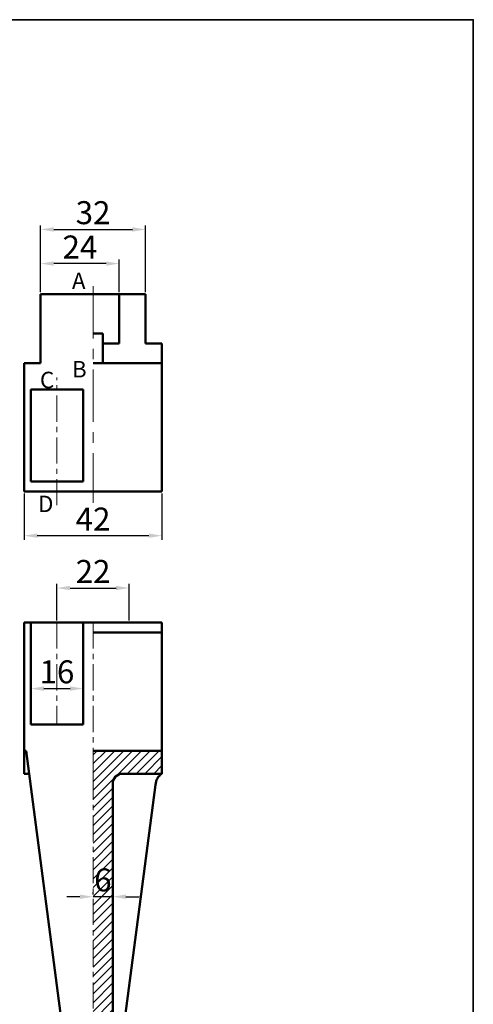
# Model space of a CAD drawing. Units: millimetres. Extents: x 214 to 813, y -258 to 321.
# Tile 4 of 4: x 674 to 813, y 22 to 321. Entities that reach past the tile are written whole.
import ezdxf

# ---------------------------------------------------------------- set-up
doc = ezdxf.new("R2010")
doc.units = ezdxf.units.MM
doc.header["$LTSCALE"] = 0.5
doc.linetypes.add('CENTER', pattern=[50.8, 31.75, -6.35, 6.35, -6.35])
for name, color, linetype, lineweight in [('M-CNTR', 1, 'CENTER', 18), ('M-DIMS', 2, 'Continuous', 25), ('M-HATC', 8, 'Continuous', 18), ('M-OUTL', 7, 'Continuous', 50), ('M-TEXT', 3, 'Continuous', 25), ('M-TTLB', 7, 'Continuous', 35)]:
    doc.layers.add(name, color=color, linetype=linetype, lineweight=lineweight)
doc.styles.get("Standard").update_dxf_attribs({"font": 'arial.ttf'})
doc.dimstyles.new('ISO-25', dxfattribs={"dimtxt": 7, "dimasz": 4, "dimexe": 1.25, "dimexo": 0.625, "dimtad": 1, "dimtoh": 1, "dimtxsty": 'Standard', "dimcen": 2.5, "dimadec": 0, "dimazin": 0, "dimtfac": 1, "dimtmove": 0, "dimatfit": 3, "dimfxl": 1, "dimarcsym": 0})

# ---------------------------------------------------------------- blocks, each defined once
blk = doc.blocks.new('*U58')
at = {"layer": 'M-CNTR', "color": 0, "transparency": 16777216}
blk.add_line((0, 41.44), (0, -24.5), dxfattribs=at)
blk = doc.blocks.new('*D59')
at = {"layer": 'Defpoints', "color": 0, "ltscale": 0.5, "transparency": 16777216}
for p in [(707.86, 148.54), (685.86, 138.04), (707.86, 138.04)]:
    blk.add_point(p, dxfattribs=at)
at = {"layer": 'M-DIMS', "color": 0, "lineweight": -2, "ltscale": 0.5, "transparency": 16777216}
for p, q in [((685.86, 138.67), (685.86, 149.79)), ((689.86, 148.54), (703.86, 148.54)), ((707.86, 138.67), (707.86, 149.79))]:
    blk.add_line(p, q, dxfattribs=at)
at = {"layer": 'M-DIMS', "color": 0, "ltscale": 0.5, "transparency": 16777216}
for points in [[(689.86, 149.21), (689.86, 147.88), (685.86, 148.54)], [(703.86, 149.21), (703.86, 147.88), (707.86, 148.54)]]:
    blk.add_solid(points, dxfattribs=at)
at = {"layer": 'M-DIMS', "color": 0, "ltscale": 0.5, "transparency": 16777216, "insert": (696.86, 152.68), "char_height": 7, "attachment_point": 5}
blk.add_mtext('22', dxfattribs=at)
blk = doc.blocks.new('*D60')
at = {"layer": 'Defpoints', "color": 0, "ltscale": 0.5, "transparency": 16777216}
for p in [(677.86, 117.94), (693.86, 117.94), (693.86, 117.94)]:
    blk.add_point(p, dxfattribs=at)
at = {"layer": 'M-DIMS', "color": 0, "lineweight": -2, "ltscale": 0.5, "transparency": 16777216}
for p, q in [((677.86, 118.56), (677.86, 119.19)), ((681.86, 117.94), (689.86, 117.94)), ((693.86, 118.56), (693.86, 119.19))]:
    blk.add_line(p, q, dxfattribs=at)
at = {"layer": 'M-DIMS', "color": 0, "ltscale": 0.5, "transparency": 16777216}
for points in [[(681.86, 118.6), (681.86, 117.27), (677.86, 117.94)], [(689.86, 118.6), (689.86, 117.27), (693.86, 117.94)]]:
    blk.add_solid(points, dxfattribs=at)
at = {"layer": 'M-DIMS', "color": 0, "ltscale": 0.5, "transparency": 16777216, "insert": (685.86, 122.13), "char_height": 7, "attachment_point": 5}
blk.add_mtext('16', dxfattribs=at)
blk = doc.blocks.new('*D61')
at = {"layer": 'Defpoints', "color": 0, "ltscale": 0.5, "transparency": 16777216}
for p in [(696.86, 54.6), (696.86, 54.6), (702.86, 54.6)]:
    blk.add_point(p, dxfattribs=at)
at = {"layer": 'M-DIMS', "color": 0, "lineweight": -2, "ltscale": 0.5, "transparency": 16777216}
for p, q in [((692.86, 54.6), (688.86, 54.6)), ((696.86, 55.23), (696.86, 55.85)), ((702.86, 54.6), (696.86, 54.6)), ((702.86, 55.23), (702.86, 55.85)), ((706.86, 54.6), (710.86, 54.6))]:
    blk.add_line(p, q, dxfattribs=at)
at = {"layer": 'M-DIMS', "color": 0, "ltscale": 0.5, "transparency": 16777216}
for points in [[(692.86, 55.27), (692.86, 53.94), (696.86, 54.6)], [(706.86, 55.27), (706.86, 53.94), (702.86, 54.6)]]:
    blk.add_solid(points, dxfattribs=at)
at = {"layer": 'M-DIMS', "color": 0, "ltscale": 0.5, "transparency": 16777216, "insert": (699.86, 58.8), "char_height": 7, "attachment_point": 5}
blk.add_mtext('6', dxfattribs=at)
blk = doc.blocks.new('*D66')
at = {"layer": 'Defpoints', "color": 0, "ltscale": 0.5, "transparency": 16777216}
for p in [(675.86, 177.96), (717.86, 177.96), (717.86, 164.48)]:
    blk.add_point(p, dxfattribs=at)
at = {"layer": 'M-DIMS', "color": 0, "lineweight": -2, "ltscale": 0.5, "transparency": 16777216}
for p, q in [((675.86, 177.34), (675.86, 163.23)), ((717.86, 177.34), (717.86, 163.23)), ((679.86, 164.48), (713.86, 164.48))]:
    blk.add_line(p, q, dxfattribs=at)
at = {"layer": 'M-DIMS', "color": 0, "ltscale": 0.5, "transparency": 16777216}
for points in [[(679.86, 165.14), (679.86, 163.81), (675.86, 164.48)], [(713.86, 165.14), (713.86, 163.81), (717.86, 164.48)]]:
    blk.add_solid(points, dxfattribs=at)
at = {"layer": 'M-DIMS', "color": 0, "ltscale": 0.5, "transparency": 16777216, "insert": (696.86, 168.62), "char_height": 7, "attachment_point": 5}
blk.add_mtext('42', dxfattribs=at)
blk = doc.blocks.new('*D67')
at = {"layer": 'Defpoints', "color": 0, "ltscale": 0.5, "transparency": 16777216}
for p in [(712.86, 257.66), (680.86, 237.96), (712.86, 237.96)]:
    blk.add_point(p, dxfattribs=at)
at = {"layer": 'M-DIMS', "color": 0, "lineweight": -2, "ltscale": 0.5, "transparency": 16777216}
for p, q in [((680.86, 238.59), (680.86, 258.91)), ((712.86, 238.59), (712.86, 258.91)), ((684.86, 257.66), (708.86, 257.66))]:
    blk.add_line(p, q, dxfattribs=at)
at = {"layer": 'M-DIMS', "color": 0, "ltscale": 0.5, "transparency": 16777216}
for points in [[(684.86, 258.33), (684.86, 256.99), (680.86, 257.66)], [(708.86, 258.33), (708.86, 256.99), (712.86, 257.66)]]:
    blk.add_solid(points, dxfattribs=at)
at = {"layer": 'M-DIMS', "color": 0, "ltscale": 0.5, "transparency": 16777216, "insert": (696.86, 261.86), "char_height": 7, "attachment_point": 5}
blk.add_mtext('32', dxfattribs=at)
blk = doc.blocks.new('*D68')
at = {"layer": 'Defpoints', "color": 0, "ltscale": 0.5, "transparency": 16777216}
for p in [(680.86, 247.28), (680.86, 237.96), (704.86, 237.96)]:
    blk.add_point(p, dxfattribs=at)
at = {"layer": 'M-DIMS', "color": 0, "lineweight": -2, "ltscale": 0.5, "transparency": 16777216}
for p, q in [((680.86, 238.59), (680.86, 248.53)), ((700.86, 247.28), (684.86, 247.28)), ((704.86, 238.59), (704.86, 248.53))]:
    blk.add_line(p, q, dxfattribs=at)
at = {"layer": 'M-DIMS', "color": 0, "ltscale": 0.5, "transparency": 16777216}
for points in [[(684.86, 247.94), (684.86, 246.61), (680.86, 247.28)], [(700.86, 247.94), (700.86, 246.61), (704.86, 247.28)]]:
    blk.add_solid(points, dxfattribs=at)
at = {"layer": 'M-DIMS', "color": 0, "ltscale": 0.5, "transparency": 16777216, "insert": (692.86, 251.41), "char_height": 7, "attachment_point": 5}
blk.add_mtext('24', dxfattribs=at)

msp = doc.modelspace()

# ---------------------------------------------------------------- hatches: boundary and pattern name
at = {"layer": 'M-HATC', "ltscale": 0.5}
h = msp.add_hatch(dxfattribs=at)
h.set_pattern_fill('ANSI31', color=256, scale=0.6)
h.set_pattern_definition([(45, (-63.675, 1e-14), (-1.3470384, 1.3470384), [])])
h.paths.add_polyline_path([(696.86, 1.042), (709.36, 1.042), (709.36, 9.042), (705.86, 9.042, -0.4142136), (702.86, 12.042), (702.86, 89.042, -0.4142136), (705.86, 92.042), (717.86, 92.042), (717.86, 99.042), (696.86, 99.042), (696.86, 92.042)])
h.paths.add_polyline_path([(696.86, -12.958), (696.86, -20.958), (709.36, -20.958), (709.36, -12.958)])

# ---------------------------------------------------------------- linework, layer by layer
at = {"layer": 'M-CNTR', "ltscale": 0.5}
for p, q in [((685.86, 173.75), (685.86, 212.593)), ((685.86, 138.042), (685.86, 107.042)), ((696.86, 138.042), (696.86, 92.042)), ((696.86, 92.042), (696.86, -31.942))]:
    msp.add_line(p, q, dxfattribs=at)
at = {"layer": 'M-OUTL', "ltscale": 0.5}
for p, q in [((712.86, 237.962), (680.86, 237.962)), ((680.86, 237.962), (680.86, 216.962)), ((704.86, 237.962), (704.86, 222.962)), ((712.86, 237.962), (712.86, 222.962)), ((699.86, 222.962), (704.86, 222.962)), ((699.86, 222.962), (704.86, 222.962)), ((712.86, 222.962), (717.86, 222.962)), ((717.86, 177.962), (717.86, 222.962)), ((675.86, 216.962), (675.86, 177.962)), ((675.86, 216.962), (680.86, 216.962)), ((696.86, 216.962), (717.86, 216.962)), ((677.86, 208.962), (693.86, 208.962)), ((677.86, 180.962), (677.86, 208.962)), ((693.86, 180.962), (693.86, 208.962)), ((677.86, 180.962), (693.86, 180.962)), ((675.86, 177.962), (717.86, 177.962)), ((675.86, 138.042), (717.86, 138.042)), ((675.86, 138.042), (675.86, 92.042)), ((677.86, 138.042), (677.86, 107.042)), ((693.86, 138.042), (693.86, 107.042)), ((717.86, 138.042), (717.86, 92.042)), ((696.86, 135.042), (717.86, 135.042)), ((677.86, 107.042), (693.86, 107.042)), ((675.86, 99.042), (676.438, 99.042)), ((676.438, 99.042), (688.528, 6.956)), ((696.86, 99.042), (717.86, 99.042)), ((675.86, 92.042), (677.357, 92.042)), ((705.86, 92.042), (717.86, 92.042)), ((702.86, 89.042), (702.86, 12.042)), ((715.923, 88.687), (705.87, 12.115))]:
    msp.add_line(p, q, dxfattribs=at)
at = {"layer": 'M-OUTL'}
for p, q in [((699.86, 225.962), (696.86, 225.962)), ((699.86, 216.962), (699.86, 225.962))]:
    msp.add_line(p, q, dxfattribs=at)
at = {"layer": 'M-OUTL', "ltscale": 0.5}
for centre, radius, start in [((705.86, 89.042), 3, 90), ((719.797, 88.687), 3.874, 120)]:
    msp.add_arc(centre, radius, start, 180, dxfattribs=at)
at = {"layer": 'M-TTLB', "ltscale": 0.5}
msp.add_lwpolyline([(214.186, 321.5), (812.717, 321.5), (812.717, -258.089), (214.186, -258.089)], close=True, dxfattribs=at)

# ---------------------------------------------------------------- block references
at = {"layer": 'M-CNTR'}
msp.add_blockref('*U58', (696.86, 198.962), dxfattribs=at)

# ---------------------------------------------------------------- texts
at = {"layer": 'M-TEXT', "ltscale": 0.5, "char_height": 5, "attachment_point": 1}
for s, insert in [('A', (690.423, 244.516)), ('B', (690.423, 217.625)), ('C', (680.675, 214.359)), ('D', (680.088, 176.64))]:
    msp.add_mtext_dynamic_manual_height_columns(s, width=7.54865, gutter_width=12.5, heights=[0], dxfattribs=dict(at, insert=insert))

# ---------------------------------------------------------------- dimensions: what is measured, and where the dimension line sits
at = {"layer": 'M-DIMS', "ltscale": 0.5}
for base, p1, p2, picture, middle in [((712.86, 257.661), (680.86, 237.962), (712.86, 237.962), '*D67', (696.86, 257.661)), ((680.86, 247.275), (704.86, 237.962), (680.86, 237.962), '*D68', (692.86, 247.275))]:
    dim = msp.add_linear_dim(base=base, p1=p1, p2=p2, dimstyle='ISO-25', override={"dimclrd": 0, "dimclre": 0, "dimclrt": 0}, dxfattribs=at)
    dim.commit()
    dim.dimension.update_dxf_attribs({"geometry": picture, "text_midpoint": middle, "dimtype": 160})
for base, p1, p2, picture, middle in [((717.86, 164.477), (675.86, 177.962), (717.86, 177.962), '*D66', (696.86, 168.617)), ((707.86, 148.543), (685.86, 138.042), (707.86, 138.042), '*D59', (696.86, 152.683)), ((693.86, 117.935), (677.86, 117.935), (693.86, 117.935), '*D60', (685.86, 122.134)), ((696.86, 54.603), (702.86, 54.603), (696.86, 54.603), '*D61', (699.86, 58.802))]:
    dim = msp.add_linear_dim(base=base, p1=p1, p2=p2, dimstyle='ISO-25', override={"dimclrd": 0, "dimclre": 0, "dimclrt": 0}, dxfattribs=at)
    dim.commit()
    dim.dimension.update_dxf_attribs({"geometry": picture, "text_midpoint": middle})

doc.saveas('drawing.dxf')
